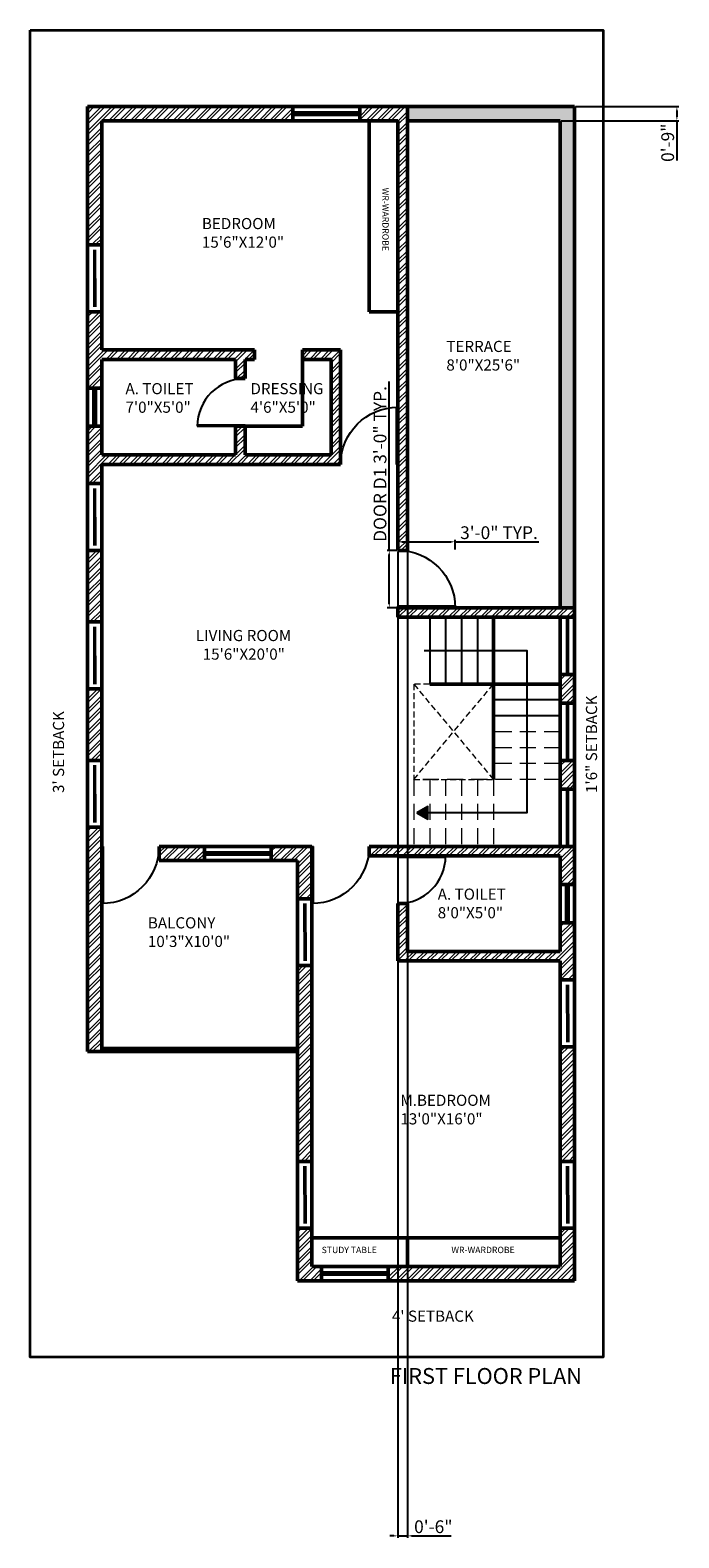
# Model space of a CAD drawing. Units: inches. Extents: x 1986 to 21484, y -1816 to 2016.
# Tile 80 of 85: x 3997 to 4404, y 953 to 1901. Entities that reach past the tile are written whole.
import ezdxf

# ---------------------------------------------------------------- set-up
doc = ezdxf.new("R2010")
doc.units = ezdxf.units.IN
doc.linetypes.add('DASHED', pattern=[19.05, 12.7, -6.35])
for name, color, linetype, lineweight in [('A-ANNO-DIMS', 2, 'Continuous', 18), ('A-ANNO-TEXT', 7, 'Continuous', 18), ('A-AREA-IDEN', 3, 'Continuous', 18), ('A-DOOR', 3, 'Continuous', 25), ('A-FLOR-STRS', 7, 'Continuous', 25), ('A-FLOR-STRS-OVHD', 8, 'DASHED', 18), ('A-GLAZ', 4, 'Continuous', 25), ('A-WALL', 7, 'Continuous', 50), ('A-WALL-PATT', 8, 'Continuous', 13), ('C-PROP', 7, 'Continuous', 35)]:
    doc.layers.add(name, color=color, linetype=linetype, lineweight=lineweight)
doc.styles.get("Standard").update_dxf_attribs({"font": 'arial.ttf'})
doc.dimstyles.new('ISO-25', dxfattribs={"dimtxt": 8, "dimasz": 2.5, "dimexe": 1.25, "dimexo": 0.625, "dimtad": 1, "dimdec": 1, "dimlunit": 3, "dimtxsty": 'Standard', "dimcen": 2.5, "dimadec": 0, "dimazin": 0, "dimtfac": 1, "dimtdec": 1, "dimtmove": 0, "dimatfit": 3, "dimfxl": 1, "dimarcsym": 0})

# ---------------------------------------------------------------- blocks, each defined once
blk = doc.blocks.new('D2')
for p, q in [((1722.5, 1505.46), (1722.5, 1475.46)), ((1723.5, 1505.46), (1723.5, 1475.46)), ((1722.5, 1475.46), (1723.5, 1475.46))]:
    blk.add_line(p, q)
blk.add_arc((1722.5, 1475.46), 30, 0, 90)
blk = doc.blocks.new('D1')
for p, q in [((1805.96, 1500.36), (1805.96, 1464.36)), ((1806.96, 1500.36), (1806.96, 1464.36)), ((1805.96, 1464.36), (1806.96, 1464.36))]:
    blk.add_line(p, q)
blk.add_arc((1805.96, 1464.36), 36, 0, 90)
blk = doc.blocks.new('WIN-36')
for p, q in [((0, 36), (0, 0)), ((0, 36), (0, 0)), ((1, 36), (1, 0))]:
    blk.add_line(p, q)
blk = doc.blocks.new('*D89')
at = {"layer": 'A-ANNO-DIMS', "color": 0, "lineweight": -2, "transparency": 16777216}
for p, q in [((4222.5, 1573.75), (4222.5, 1679.89)), ((4227.28, 1573.75), (4221.25, 1573.75)), ((4222.5, 1540.25), (4222.5, 1571.25)), ((4227.28, 1537.75), (4221.25, 1537.75))]:
    blk.add_line(p, q, dxfattribs=at)
at = {"layer": 'A-ANNO-DIMS', "color": 0, "transparency": 16777216}
for points in [[(4222.08, 1571.25), (4222.92, 1571.25), (4222.5, 1573.75)], [(4222.08, 1540.25), (4222.92, 1540.25), (4222.5, 1537.75)]]:
    blk.add_solid(points, dxfattribs=at)
at = {"layer": 'Defpoints', "color": 0, "transparency": 16777216}
for p in [(4222.5, 1573.75), (4227.9, 1573.75), (4227.9, 1537.75)]:
    blk.add_point(p, dxfattribs=at)
at = {"layer": 'A-ANNO-DIMS', "color": 0, "transparency": 16777216, "insert": (4217.73, 1628.07), "char_height": 8, "attachment_point": 5, "rotation": 90}
blk.add_mtext('DOOR D1 3\'-0" TYP.', dxfattribs=at)
blk = doc.blocks.new('*D90')
at = {"layer": 'A-ANNO-DIMS', "color": 0, "lineweight": -2, "transparency": 16777216}
for p, q in [((4227.9, 1574.38), (4227.9, 1580.4)), ((4230.4, 1579.15), (4261.4, 1579.15)), ((4263.9, 1574.38), (4263.9, 1580.4)), ((4263.9, 1579.15), (4316.41, 1579.15))]:
    blk.add_line(p, q, dxfattribs=at)
at = {"layer": 'A-ANNO-DIMS', "color": 0, "transparency": 16777216}
for points in [[(4230.4, 1579.57), (4230.4, 1578.74), (4227.9, 1579.15)], [(4261.4, 1579.57), (4261.4, 1578.74), (4263.9, 1579.15)]]:
    blk.add_solid(points, dxfattribs=at)
at = {"layer": 'Defpoints', "color": 0, "transparency": 16777216}
for p in [(4227.9, 1573.75), (4263.9, 1579.15), (4263.9, 1573.75)]:
    blk.add_point(p, dxfattribs=at)
at = {"layer": 'A-ANNO-DIMS', "color": 0, "transparency": 16777216, "insert": (4291.41, 1583.86), "char_height": 8, "attachment_point": 5}
blk.add_mtext('3\'-0" TYP.', dxfattribs=at)
blk = doc.blocks.new('*D129')
at = {"layer": 'A-ANNO-DIMS', "color": 0, "lineweight": -2, "transparency": 16777216}
for p, q in [((4339.53, 1852.75), (4404.4, 1852.75)), ((4403.15, 1850.25), (4403.15, 1846.25)), ((4330.53, 1843.75), (4404.4, 1843.75)), ((4403.15, 1843.75), (4403.15, 1818.74))]:
    blk.add_line(p, q, dxfattribs=at)
at = {"layer": 'A-ANNO-DIMS', "color": 0, "transparency": 16777216}
for points in [[(4402.73, 1850.25), (4403.57, 1850.25), (4403.15, 1852.75)], [(4402.73, 1846.25), (4403.57, 1846.25), (4403.15, 1843.75)]]:
    blk.add_solid(points, dxfattribs=at)
at = {"layer": 'Defpoints', "color": 0, "transparency": 16777216}
for p in [(4338.9, 1852.75), (4329.9, 1843.75), (4403.15, 1843.75)]:
    blk.add_point(p, dxfattribs=at)
at = {"layer": 'A-ANNO-DIMS', "color": 0, "transparency": 16777216, "insert": (4398.44, 1829.99), "char_height": 8, "attachment_point": 5, "rotation": 90}
blk.add_mtext('0\'-9"', dxfattribs=at)
blk = doc.blocks.new('*D130')
at = {"layer": 'A-ANNO-DIMS', "color": 0, "lineweight": -2, "transparency": 16777216}
for p, q in [((4227.9, 1573.13), (4227.9, 953.11)), ((4233.9, 1573.13), (4233.9, 953.11)), ((4225.4, 954.36), (4222.9, 954.36)), ((4227.9, 954.36), (4233.9, 954.36)), ((4236.4, 954.36), (4261.42, 954.36))]:
    blk.add_line(p, q, dxfattribs=at)
at = {"layer": 'A-ANNO-DIMS', "color": 0, "transparency": 16777216}
for points in [[(4225.4, 954.78), (4225.4, 953.95), (4227.9, 954.36)], [(4236.4, 954.78), (4236.4, 953.95), (4233.9, 954.36)]]:
    blk.add_solid(points, dxfattribs=at)
at = {"layer": 'Defpoints', "color": 0, "transparency": 16777216}
for p in [(4227.9, 1573.75), (4233.9, 1573.75), (4233.9, 954.36)]:
    blk.add_point(p, dxfattribs=at)
at = {"layer": 'A-ANNO-DIMS', "color": 0, "transparency": 16777216, "insert": (4250.16, 959.07), "char_height": 8, "attachment_point": 5}
blk.add_mtext('0\'-6"', dxfattribs=at)

msp = doc.modelspace()

# ---------------------------------------------------------------- hatches: boundary and pattern name
at = {"layer": 'A-FLOR-STRS'}
h = msp.add_hatch(color=256, dxfattribs=at)
h.dxf.hatch_style = 1
h.paths.add_polyline_path([(4239.74, 1408.75), (4246.69, 1404.74), (4246.69, 1412.77)])
at = {"layer": 'A-WALL-PATT'}
h = msp.add_hatch(dxfattribs=at)
h.set_pattern_fill('ANSI32', color=256, scale=0.5)
h.paths.add_polyline_path([(4161.9, 1852.75), (4032.9, 1852.75), (4032.9, 1765.75), (4041.9, 1765.75), (4041.9, 1843.75), (4161.9, 1843.75)])
h.paths.add_polyline_path([(4137.9, 1699.75), (4041.9, 1699.75), (4041.9, 1723.75), (4032.9, 1723.75), (4032.9, 1675.75), (4041.9, 1675.75), (4041.9, 1693.75), (4125.9, 1693.75), (4125.9, 1681.75), (4131.9, 1681.75), (4131.9, 1693.75), (4137.9, 1693.75)])
h.paths.add_polyline_path([(4233.9, 1852.75), (4203.9, 1852.75), (4203.9, 1843.75), (4227.9, 1843.75), (4227.9, 1573.75), (4233.9, 1573.75)])
h.paths.add_polyline_path([(4041.9, 1651.75), (4032.9, 1651.75), (4032.9, 1615.75), (4041.9, 1615.75), (4041.9, 1627.75), (4191.9, 1627.75), (4191.9, 1699.75), (4167.9, 1699.75), (4167.9, 1693.75), (4185.9, 1693.75), (4185.9, 1633.75), (4131.9, 1633.75), (4131.9, 1651.75), (4125.9, 1651.75), (4125.9, 1633.75), (4041.9, 1633.75)])
h.paths.add_polyline_path([(4041.9, 1573.75), (4032.9, 1573.75), (4032.9, 1528.77), (4041.9, 1528.77)])
h.paths.add_polyline_path([(4041.9, 1486.77), (4032.9, 1486.77), (4032.9, 1441.75), (4041.9, 1441.75)])
h.paths.add_polyline_path([(4041.9, 1399.75), (4032.9, 1399.75), (4032.9, 1258.75), (4041.9, 1258.75)])
h.paths.add_polyline_path([(4106.4, 1387.75), (4077.9, 1387.75), (4077.9, 1378.75), (4106.4, 1378.75)])
h.paths.add_polyline_path([(4173.9, 1387.75), (4148.4, 1387.75), (4148.4, 1378.75), (4164.9, 1378.75), (4164.9, 1354.75), (4173.9, 1354.75)])
h.paths.add_polyline_path([(4338.9, 1387.75), (4329.9, 1387.75), (4209.9, 1387.75), (4209.9, 1381.75), (4329.9, 1381.75), (4329.9, 1363.75), (4338.9, 1363.75)])
h.paths.add_polyline_path([(4338.9, 1495.75), (4329.9, 1495.75), (4329.9, 1477.75), (4338.9, 1477.75)])
h.paths.add_polyline_path([(4338.9, 1537.75), (4227.9, 1537.75), (4227.9, 1531.75), (4329.9, 1531.75), (4338.9, 1531.75)])
h.paths.add_polyline_path([(4338.9, 1441.75), (4329.9, 1441.75), (4329.9, 1423.75), (4338.9, 1423.75)])
h.paths.add_polyline_path([(4338.9, 1339.75), (4329.9, 1339.75), (4329.9, 1321.75), (4233.9, 1321.75), (4233.9, 1351.75), (4227.9, 1351.75), (4227.9, 1315.75), (4329.9, 1315.75), (4329.9, 1303.75), (4338.9, 1303.75)])
h.paths.add_polyline_path([(4338.9, 1261.75), (4329.9, 1261.75), (4329.9, 1189.75), (4338.9, 1189.75)])
h.paths.add_polyline_path([(4338.9, 1147.75), (4329.9, 1147.75), (4329.9, 1123.75), (4221.9, 1123.75), (4221.9, 1114.75), (4338.9, 1114.75)])
h.paths.add_polyline_path([(4173.9, 1147.75), (4164.9, 1147.75), (4164.9, 1114.75), (4179.9, 1114.75), (4179.9, 1123.75), (4173.9, 1123.75)])
h.paths.add_polyline_path([(4173.9, 1312.75), (4164.9, 1312.75), (4164.9, 1189.75), (4173.9, 1189.75)])
h = msp.add_hatch(color=256, dxfattribs=at)
h.dxf.hatch_style = 1
h.paths.add_polyline_path([(4338.9, 1852.75), (4233.9, 1852.75), (4233.9, 1843.75), (4329.9, 1843.75), (4329.9, 1537.75), (4338.9, 1537.75)])

# ---------------------------------------------------------------- linework, layer by layer
at = {"layer": 'A-FLOR-STRS'}
for p, q in [((4247.9, 1531.75), (4247.9, 1489.75)), ((4257.9, 1531.75), (4257.9, 1489.75)), ((4267.9, 1531.75), (4267.9, 1489.75)), ((4277.9, 1531.75), (4277.9, 1489.75)), ((4329.9, 1479.75), (4287.9, 1479.75)), ((4329.9, 1469.75), (4287.9, 1469.75))]:
    msp.add_line(p, q, dxfattribs=at)
msp.add_lwpolyline([(4244.49, 1510.75), (4308.9, 1510.75), (4308.9, 1408.75), (4246.69, 1408.75)], dxfattribs=at)
msp.add_lwpolyline([(4239.74, 1408.75), (4246.69, 1404.74), (4246.69, 1412.77)], close=True, dxfattribs=at)
at = {"layer": 'A-FLOR-STRS-OVHD', "ltscale": 0.3}
for p, q in [((4237.9, 1489.75), (4287.9, 1429.75)), ((4237.9, 1429.75), (4287.9, 1489.75))]:
    msp.add_line(p, q, dxfattribs=at)
at = {"layer": 'A-FLOR-STRS-OVHD', "ltscale": 0.8}
for p, q in [((4329.9, 1459.75), (4287.9, 1459.75)), ((4329.9, 1449.75), (4287.9, 1449.75)), ((4329.9, 1439.75), (4287.9, 1439.75)), ((4237.9, 1429.75), (4237.9, 1387.75)), ((4329.9, 1429.75), (4237.9, 1429.75)), ((4247.9, 1429.75), (4247.9, 1387.75)), ((4257.9, 1429.75), (4257.9, 1387.75)), ((4267.9, 1429.75), (4267.9, 1387.75)), ((4277.9, 1429.75), (4277.9, 1387.75)), ((4287.9, 1429.75), (4287.9, 1387.75))]:
    msp.add_line(p, q, dxfattribs=at)
at = {"layer": 'A-FLOR-STRS-OVHD', "ltscale": 0.3}
msp.add_lwpolyline([(4237.9, 1429.75), (4287.9, 1429.75), (4287.9, 1489.75), (4237.9, 1489.75)], close=True, dxfattribs=at)
at = {"layer": 'A-WALL'}
for p, q in [((4032.9, 1852.75), (4338.9, 1852.75)), ((4032.9, 1258.75), (4032.9, 1852.75)), ((4161.9, 1843.75), (4161.9, 1852.75)), ((4161.9, 1848.75), (4203.9, 1848.75)), ((4203.9, 1843.75), (4203.9, 1852.75)), ((4233.9, 1852.75), (4233.9, 1573.75)), ((4338.9, 1852.75), (4338.9, 1114.75)), ((4041.9, 1843.75), (4227.9, 1843.75)), ((4041.9, 1699.75), (4041.9, 1843.75)), ((4161.9, 1847.75), (4203.9, 1847.75)), ((4209.9, 1843.75), (4209.9, 1723.75)), ((4227.9, 1843.75), (4227.9, 1573.75)), ((4233.9, 1843.75), (4329.9, 1843.75)), ((4329.9, 1843.75), (4329.9, 1537.75)), ((4032.9, 1765.75), (4041.9, 1765.75)), ((4032.9, 1723.75), (4041.9, 1723.75)), ((4209.9, 1723.75), (4227.9, 1723.75)), ((4041.9, 1699.75), (4137.9, 1699.75)), ((4137.9, 1699.75), (4137.9, 1693.75)), ((4167.9, 1699.75), (4191.9, 1699.75)), ((4167.9, 1699.75), (4167.9, 1651.75)), ((4191.9, 1699.75), (4191.9, 1627.75)), ((4041.9, 1693.75), (4125.9, 1693.75)), ((4041.9, 1633.75), (4041.9, 1693.75)), ((4125.9, 1681.75), (4125.9, 1693.75)), ((4131.9, 1693.75), (4137.9, 1693.75)), ((4131.9, 1681.75), (4131.9, 1693.75)), ((4167.9, 1693.75), (4185.9, 1693.75)), ((4185.9, 1693.75), (4185.9, 1633.75)), ((4125.9, 1681.75), (4131.9, 1681.75)), ((4032.9, 1675.75), (4041.9, 1675.75)), ((4036.9, 1651.75), (4036.9, 1675.75)), ((4037.9, 1651.75), (4037.9, 1675.75)), ((4032.9, 1651.75), (4041.9, 1651.75)), ((4125.9, 1633.75), (4125.9, 1651.75)), ((4125.9, 1651.75), (4167.9, 1651.75)), ((4131.9, 1633.75), (4131.9, 1651.75)), ((4041.9, 1633.75), (4125.9, 1633.75)), ((4131.9, 1633.75), (4185.9, 1633.75)), ((4041.9, 1258.75), (4041.9, 1627.75)), ((4041.9, 1627.75), (4191.9, 1627.75)), ((4032.9, 1615.75), (4041.9, 1615.75)), ((4032.9, 1573.75), (4041.9, 1573.75)), ((4227.9, 1573.75), (4233.9, 1573.75)), ((4227.9, 1537.75), (4338.9, 1537.75)), ((4227.9, 1537.75), (4227.9, 1531.75)), ((4032.9, 1528.77), (4041.9, 1528.77)), ((4227.9, 1531.75), (4329.9, 1531.75)), ((4287.9, 1531.75), (4287.9, 1429.75)), ((4329.9, 1531.75), (4329.9, 1387.75)), ((4329.9, 1531.75), (4338.9, 1531.75)), ((4329.9, 1489.75), (4247.9, 1489.75)), ((4329.9, 1495.75), (4338.9, 1495.75)), ((4032.9, 1486.77), (4041.9, 1486.77)), ((4329.9, 1477.75), (4338.9, 1477.75)), ((4032.9, 1441.75), (4041.9, 1441.75)), ((4329.9, 1441.75), (4338.9, 1441.75)), ((4329.9, 1423.75), (4338.9, 1423.75)), ((4032.9, 1399.75), (4041.9, 1399.75)), ((4077.9, 1378.75), (4077.9, 1387.75)), ((4077.9, 1387.75), (4173.9, 1387.75)), ((4106.4, 1378.75), (4106.4, 1387.75)), ((4106.4, 1383.75), (4148.4, 1383.75)), ((4148.4, 1378.75), (4148.4, 1387.75)), ((4173.9, 1123.75), (4173.9, 1387.75)), ((4209.9, 1387.75), (4329.9, 1387.75)), ((4209.9, 1381.75), (4209.9, 1387.75)), ((4329.9, 1387.75), (4338.9, 1387.75)), ((4077.9, 1378.75), (4164.9, 1378.75)), ((4106.4, 1382.75), (4148.4, 1382.75)), ((4164.9, 1114.75), (4164.9, 1378.75)), ((4209.9, 1381.75), (4329.9, 1381.75)), ((4329.9, 1381.75), (4329.9, 1321.75)), ((4329.9, 1363.75), (4338.9, 1363.75)), ((4333.9, 1339.75), (4333.9, 1363.75)), ((4334.9, 1339.75), (4334.9, 1363.75)), ((4164.9, 1354.75), (4173.9, 1354.75)), ((4227.9, 1351.75), (4227.9, 1315.75)), ((4227.9, 1351.75), (4233.9, 1351.75)), ((4233.9, 1351.75), (4233.9, 1321.75)), ((4329.9, 1339.75), (4338.9, 1339.75)), ((4233.9, 1321.75), (4329.9, 1321.75)), ((4164.9, 1312.75), (4173.9, 1312.75)), ((4227.9, 1315.75), (4329.9, 1315.75)), ((4329.9, 1315.75), (4329.9, 1123.75)), ((4329.9, 1303.75), (4338.9, 1303.75)), ((4041.9, 1260.75), (4164.9, 1260.75)), ((4329.9, 1261.75), (4338.9, 1261.75)), ((4032.9, 1258.75), (4164.9, 1258.75)), ((4164.9, 1189.75), (4173.9, 1189.75)), ((4329.9, 1189.75), (4338.9, 1189.75)), ((4164.9, 1147.75), (4173.9, 1147.75)), ((4329.9, 1147.75), (4338.9, 1147.75)), ((4173.9, 1141.75), (4329.9, 1141.75)), ((4233.9, 1123.75), (4233.9, 1141.75)), ((4233.9, 1123.75), (4233.9, 1141.75)), ((4173.9, 1123.75), (4329.9, 1123.75)), ((4179.9, 1114.75), (4179.9, 1123.75)), ((4179.9, 1119.75), (4221.9, 1119.75)), ((4179.9, 1118.75), (4221.9, 1118.75)), ((4221.9, 1114.75), (4221.9, 1123.75)), ((4338.9, 1114.75), (4164.9, 1114.75))]:
    msp.add_line(p, q, dxfattribs=at)
at = {"layer": 'C-PROP'}
msp.add_lwpolyline([(3996.9, 1900.75), (4356.9, 1900.75), (4356.9, 1066.75), (3996.9, 1066.75)], close=True, dxfattribs=at)

# ---------------------------------------------------------------- block references
at = {"layer": 'A-DOOR'}
for p, rotation in [((5607.36, -70.75), 90), ((2752.44, 3104.25), 270)]:
    msp.add_blockref('D2', p, dxfattribs=dict(at, rotation=rotation))
at = {"layer": 'A-DOOR', "xscale": -1}
msp.add_blockref('D1', (6033.87, 163.39), dxfattribs=at)
for p, rotation in [((2763.54, -268.21), 270), ((2235.94, 2852.11), 180), ((2367.94, 2852.11), 180)]:
    msp.add_blockref('D1', p, dxfattribs=dict(at, rotation=rotation))
at = {"layer": 'A-GLAZ'}
for p, rotation in [((4037, 1726.75), 0.3027934322096833), ((4037, 1576.75), 0.3027934322120907), ((4037, 1489.77), 0.3027934322096833), ((4037, 1402.75), 0.3027934322048686), ((4169, 1315.75), 0.302793432207276), ((4334, 1264.75), 0.302793432207276), ((4169, 1150.75), 0.302793432207276), ((4334, 1150.75), 0.302793432207276)]:
    msp.add_blockref('WIN-36', p, dxfattribs=dict(at, rotation=rotation))
for p in [(4333.9, 1495.75), (4333.9, 1441.75), (4333.9, 1387.75)]:
    msp.add_blockref('WIN-36', p, dxfattribs=at)

# ---------------------------------------------------------------- texts
at = {"layer": 'A-ANNO-TEXT', "attachment_point": 1}
for s, insert, char_height, rotation in [('{\\fTimes New Roman|b0|i0|c0|p18;WR-WARDROBE}', (4222.16, 1801.73), 4, 270), ('{\\fTimes New Roman|b0|i0|c0|p18;1\'6" SETBACK}', (4346.04, 1421.26), 7, 90), ("{\\fTimes New Roman|b0|i0|c0|p18;3' SETBACK}", (4011.21, 1421.26), 7, 90)]:
    msp.add_mtext_dynamic_manual_height_columns(s, width=105.6127, gutter_width=12.5, heights=[0], dxfattribs=dict(at, insert=insert, char_height=char_height, rotation=rotation))
for s, width, insert, char_height in [('{\\fTimes New Roman|b0|i0|c0|p18;STUDY TABLE}', 105.6127, (4180.01, 1136.07), 4), ('{\\fTimes New Roman|b0|i0|c0|p18;WR-WARDROBE}', 105.6127, (4261.52, 1136.07), 4), ("{\\fTimes New Roman|b0|i0|c0|p18;4' SETBACK}", 105.6127, (4224.14, 1095.97), 7), ('{\\fTimes New Roman|b0|i0|c0|p18;FIRST FLOOR PLAN}', 226.7688, (4222.88, 1059.84), 10)]:
    msp.add_mtext_dynamic_manual_height_columns(s, width=width, gutter_width=12.5, heights=[0], dxfattribs=dict(at, insert=insert, char_height=char_height))
at = {"layer": 'A-AREA-IDEN', "char_height": 7, "attachment_point": 1}
for s, width, insert in [('{\\fTimes New Roman|b0|i0|c0|p18;BEDROOM \\P15\'6"X12\'0"}', 105.6127, (4104.79, 1782.68)), ('{\\fTimes New Roman|b0|i0|c0|p18;TERRACE\\P8\'0"X25\'6"}', 105.6127, (4258.36, 1705.47)), ('{\\fTimes New Roman|b0|i0|c0|p18;A. TOILET\\P7\'0"X5\'0"}', 105.6127, (4056.76, 1678.93)), ('{\\fTimes New Roman|b0|i0|c0|p18;DRESSING\\P4\'6"X5\'0"}', 105.6127, (4135.29, 1678.93)), ('{\\fTimes New Roman|b0|i0|c0|p18;LIVING ROOM\\P  15\'6"X20\'0"}', 122.2228, (4101.01, 1523.75)), ('{\\fTimes New Roman|b0|i0|c0|p18;A. TOILET\\P8\'0"X5\'0"}', 105.6127, (4252.94, 1361.19)), ('{\\fTimes New Roman|b0|i0|c0|p18;BALCONY\\P10\'3"X10\'0"}', 105.6127, (4070.85, 1343.16)), ('{\\fTimes New Roman|b0|i0|c0|p18;M.BEDROOM \\P13\'0"X16\'0"}', 105.6127, (4229.47, 1231.63))]:
    msp.add_mtext_dynamic_manual_height_columns(s, width=width, gutter_width=12.5, heights=[0], dxfattribs=dict(at, insert=insert))

# ---------------------------------------------------------------- dimensions: what is measured, and where the dimension line sits
at = {"layer": 'A-ANNO-DIMS'}
dim = msp.add_linear_dim(base=(4403.15, 1843.75), p1=(4338.9, 1852.75), p2=(4329.9, 1843.75), angle=90, dimstyle='ISO-25', override={"dimdec": 1, "dimlfac": 1, "dimrnd": 0, "dimzin": 1, "dimdsep": 46, "dimlunit": 4, "dimfrac": 2}, dxfattribs=at)
dim.commit()
dim.dimension.update_dxf_attribs({"geometry": '*D129', "text_midpoint": (4398.44, 1829.99)})
dim = msp.add_linear_dim(base=(4222.5, 1573.75), p1=(4227.9, 1537.75), p2=(4227.9, 1573.75), angle=90, text='DOOR D1 <> TYP.', dimstyle='ISO-25', override={"dimdec": 1, "dimrnd": 0, "dimzin": 1, "dimlunit": 4, "dimfrac": 2}, dxfattribs=at)
dim.commit()
dim.dimension.update_dxf_attribs({"geometry": '*D89', "text_midpoint": (4217.73, 1628.07)})
dim = msp.add_linear_dim(base=(4263.9, 1579.15), p1=(4227.9, 1573.75), p2=(4263.9, 1573.75), text='<> TYP.', dimstyle='ISO-25', override={"dimdec": 1, "dimrnd": 0, "dimzin": 1, "dimlunit": 4, "dimfrac": 2}, dxfattribs=at)
dim.commit()
dim.dimension.update_dxf_attribs({"geometry": '*D90', "text_midpoint": (4291.41, 1583.86)})
dim = msp.add_linear_dim(base=(4233.9, 954.36), p1=(4227.9, 1573.75), p2=(4233.9, 1573.75), dimstyle='ISO-25', override={"dimdec": 1, "dimlfac": 1, "dimrnd": 0, "dimzin": 1, "dimdsep": 46, "dimlunit": 4, "dimfrac": 2}, dxfattribs=at)
dim.commit()
dim.dimension.update_dxf_attribs({"geometry": '*D130', "text_midpoint": (4250.16, 959.07)})

doc.saveas('drawing.dxf')
